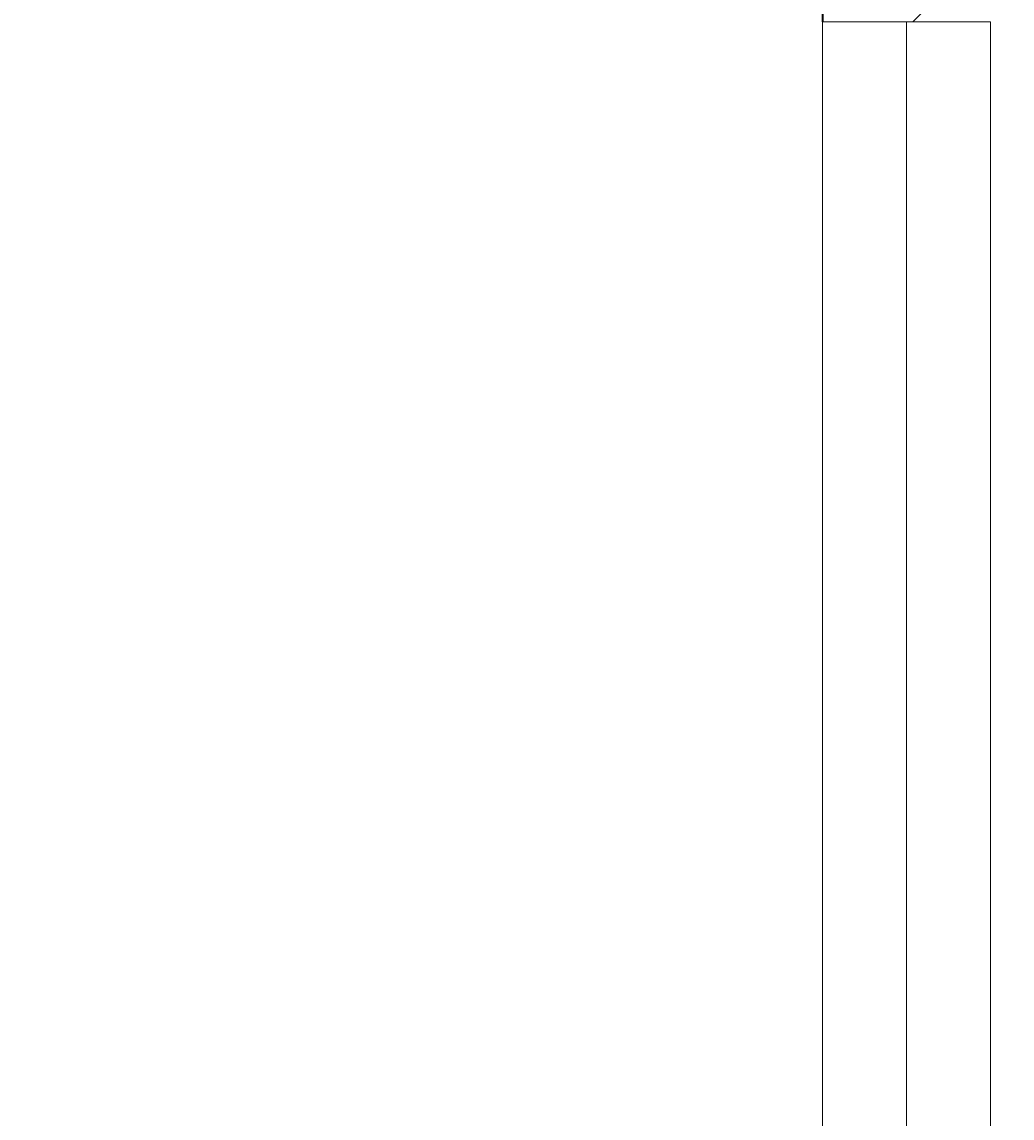
# Model space of a CAD drawing. Units: inches. Extents: x 1885 to 2748, y 783 to 2421.
# Tile 62 of 117: x 1995 to 2022, y 1949 to 1979. Entities that reach past the tile are written whole.
import ezdxf

# ---------------------------------------------------------------- set-up
doc = ezdxf.new("R2010")
doc.units = ezdxf.units.IN
for name, color, linetype, lineweight in [('A-ANNO-DIMS', 2, 'Continuous', 18), ('A-GLAZ', 181, 'Continuous', 18), ('A-WALL', 7, 'Continuous', 35)]:
    doc.layers.add(name, color=color, linetype=linetype, lineweight=lineweight)
doc.layers.add('A-WALL-PATT', color=85, linetype='Continuous', lineweight=13, true_color=0x58ba48)
doc.styles.get("Standard").update_dxf_attribs({"font": 'arial.ttf'})
doc.dimstyles.get("Standard").update_dxf_attribs({"dimtxt": 0.18, "dimasz": 0.18, "dimexe": 0.18, "dimexo": 0.0625, "dimgap": 0.09, "dimtad": 0, "dimtih": 1, "dimtoh": 1, "dimdec": 4, "dimzin": 0, "dimdsep": 46, "dimtxsty": 'Standard', "dimcen": 0.09, "dimadec": 0, "dimazin": 0, "dimtfac": 1, "dimtdec": 4, "dimtofl": 0, "dimtmove": 0, "dimatfit": 3, "dimfxl": 1, "dimtolj": 1, "dimtzin": 0, "dimarcsym": 0})

# ---------------------------------------------------------------- blocks, each defined once
blk = doc.blocks.new('WIN-60-ALT')
for p, q in [((0.004, 59.998), (4.504, 59.998)), ((0.004, 59.998), (0.004, -0.002)), ((4.504, 59.998), (2.254, 59.998)), ((2.254, 59.998), (2.254, -0.002)), ((4.504, -0.002), (4.504, 59.998))]:
    blk.add_line(p, q)
blk = doc.blocks.new('*D48')
at = {"layer": 'A-ANNO-DIMS', "color": 0, "lineweight": -2, "transparency": 16777216}
for p, q in [((1980.711, 2348.006), (1902.844, 2348.006)), ((1903.024, 2347.826), (1903.024, 2114.937)), ((1903.024, 1881.686), (1903.024, 2114.574)), ((2016.711, 1881.506), (1902.844, 1881.506))]:
    blk.add_line(p, q, dxfattribs=at)
at = {"layer": 'A-ANNO-DIMS', "color": 0, "transparency": 16777216}
for points in [[(1902.994, 2347.826), (1903.054, 2347.826), (1903.024, 2348.006)], [(1902.994, 1881.686), (1903.054, 1881.686), (1903.024, 1881.506)]]:
    blk.add_solid(points, dxfattribs=at)
at = {"layer": 'Defpoints', "color": 0, "transparency": 16777216}
for p in [(1903.024, 2348.006), (1980.774, 2348.006), (2016.774, 1881.506)]:
    blk.add_point(p, dxfattribs=at)
at = {"layer": 'A-ANNO-DIMS', "color": 0, "transparency": 16777216, "insert": (1903.024, 2114.756), "char_height": 0.18, "attachment_point": 5}
blk.add_mtext('\\A1;466.5', dxfattribs=at)

msp = doc.modelspace()

# ---------------------------------------------------------------- hatches: boundary and pattern name
at = {"layer": 'A-WALL-PATT'}
h = msp.add_hatch(dxfattribs=at)
h.set_pattern_fill('ANSI32', color=256)
h.paths.add_polyline_path([(2007.772, 2318.006), (1980.774, 2318.006), (1980.774, 2281.215), (1985.274, 2281.215), (1985.274, 2313.506), (2007.772, 2313.506), (2007.772, 2315.756)])
h.paths.add_polyline_path([(2094.324, 2318.006), (2067.772, 2318.006), (2067.772, 2313.506), (2094.324, 2313.506), (2094.324, 2315.756)])
h.paths.add_polyline_path([(2131.367, 2315.756), (2131.367, 2318.006), (2131.189, 2318.006), (2112.609, 2318.006), (2112.609, 2313.506), (2117.274, 2313.506), (2117.274, 2255.201), (2121.774, 2255.201), (2121.774, 2313.506), (2131.367, 2313.506)])
h.paths.add_polyline_path([(2190.512, 2318.006), (2155.367, 2318.006), (2155.367, 2313.506), (2169.774, 2313.506), (2169.774, 2229.506), (2121.774, 2229.506), (2121.774, 2233.451), (2119.524, 2233.451), (2117.274, 2233.451), (2117.274, 2201.101), (2121.774, 2201.101), (2121.774, 2225.006), (2169.774, 2225.006), (2169.774, 2165.006), (2306.274, 2165.006), (2306.274, 2066.006), (2310.774, 2066.006), (2344.274, 2066.006), (2486.274, 2066.006), (2486.274, 1886.006), (2483.02, 1886.006), (2483.02, 1881.506), (2486.274, 1881.506), (2486.274, 1880.678), (2490.774, 1880.678), (2490.774, 2070.506), (2344.274, 2070.506), (2310.774, 2070.506), (2310.774, 2165.006), (2310.774, 2173.636), (2308.524, 2173.636), (2306.274, 2173.636), (2306.274, 2169.506), (2174.274, 2169.506), (2174.274, 2313.506), (2190.512, 2313.506), (2190.512, 2315.756)])
h.paths.add_polyline_path([(1985.274, 2221.215), (1980.774, 2221.215), (1980.774, 2165.006), (1992.774, 2165.006), (1992.774, 2141.927), (1997.274, 2141.927), (1997.274, 2165.006), (2117.274, 2165.006), (2117.274, 2163.126), (2121.774, 2163.126), (2121.774, 2172.734), (2119.524, 2172.734), (2117.274, 2172.734), (2117.274, 2169.506), (1985.274, 2169.506)])
h.paths.add_polyline_path([(1997.274, 2105.927), (1992.774, 2105.927), (1992.774, 2070.506), (2016.774, 2070.506), (2016.774, 2059.123), (2019.024, 2059.123), (2021.274, 2059.123), (2021.274, 2070.506), (2117.274, 2070.506), (2117.274, 2022.506), (2114.423, 2022.506), (2114.423, 2018.006), (2123.627, 2018.006), (2123.627, 2020.256), (2123.627, 2022.506), (2121.774, 2022.506), (2121.774, 2142.587), (2119.524, 2142.587), (2117.274, 2142.587), (2117.274, 2075.006), (1997.274, 2075.006)])
h.paths.add_polyline_path([(2092.029, 2020.256), (2092.029, 2022.506), (2021.274, 2022.506), (2021.274, 2035.123), (2016.774, 2035.123), (2016.774, 2018.006), (2016.774, 1978.784), (2021.274, 1978.784), (2021.274, 2018.006), (2092.029, 2018.006)])
h.paths.add_polyline_path([(2260.938, 2022.506), (2153.105, 2022.506), (2153.105, 2020.256), (2153.105, 2018.006), (2155.274, 2018.006), (2155.274, 1886.006), (2107.629, 1886.006), (2107.629, 1881.506), (2182.911, 1881.506), (2182.911, 1883.756), (2182.911, 1886.006), (2159.774, 1886.006), (2159.774, 2018.006), (2260.938, 2018.006), (2260.938, 2020.256)])
h.paths.add_polyline_path([(2047.629, 1883.756), (2047.629, 1886.006), (2021.274, 1886.006), (2021.274, 1918.784), (2019.024, 1918.784), (2016.774, 1918.784), (2016.774, 1881.506), (2047.629, 1881.506)])
h.paths.add_polyline_path([(2306.361, 1883.756), (2306.361, 1886.006), (2296.274, 1886.006), (2296.274, 1982.006), (2316.535, 1982.006), (2316.535, 1984.256), (2316.535, 1986.506), (2296.274, 1986.506), (2296.274, 2022.506), (2289.276, 2022.506), (2289.276, 2018.006), (2291.774, 2018.006), (2291.774, 1886.006), (2242.911, 1886.006), (2242.911, 1881.506), (2306.361, 1881.506)], flags=17)
h.paths.add_polyline_path([(1985.274, 1843.006), (2021.6, 1843.006), (2021.534, 1845.441), (2021.477, 1847.506), (1980.774, 1847.506), (1980.774, 1809.446), (1985.274, 1809.446)])
h.paths.add_polyline_path([(2131.482, 1845.256), (2131.482, 1847.506), (2081.534, 1847.506), (2081.534, 1843.006), (2117.274, 1843.006), (2117.274, 1784.147), (2119.524, 1784.147), (2121.774, 1784.147), (2121.774, 1843.006), (2131.482, 1843.006)])
h.paths.add_polyline_path([(2203.886, 1847.506), (2155.482, 1847.506), (2155.482, 1843.006), (2169.774, 1843.006), (2169.774, 1759.006), (2121.774, 1759.006), (2121.774, 1761.457), (2117.274, 1761.457), (2117.274, 1730.429), (2121.774, 1730.429), (2121.774, 1754.506), (2177.421, 1754.506), (2177.421, 1756.756), (2177.421, 1759.006), (2174.274, 1759.006), (2174.274, 1843.006), (2203.886, 1843.006)])
h.paths.add_polyline_path([(2335.554, 1845.256), (2335.554, 1847.506), (2239.886, 1847.506), (2239.886, 1843.006), (2306.274, 1843.006), (2306.274, 1759.006), (2199.486, 1759.006), (2199.486, 1754.506), (2310.774, 1754.506), (2310.774, 1843.006), (2335.554, 1843.006)])
h.paths.add_polyline_path([(2348.774, 2022.506), (2344.274, 2022.506), (2344.274, 1986.506), (2341.681, 1986.506), (2341.681, 1982.006), (2344.274, 1982.006), (2344.274, 1886.006), (2330.361, 1886.006), (2330.361, 1881.506), (2361.627, 1881.506), (2361.627, 1883.756), (2361.627, 1886.006), (2348.774, 1886.006)], flags=17)
h.paths.add_polyline_path([(2283.251, 2315.756), (2283.251, 2318.006), (2238.512, 2318.006), (2238.512, 2313.506), (2283.251, 2313.506)], flags=17)
h.paths.add_polyline_path([(2363.274, 2348.006), (2388.677, 2348.006), (2388.677, 2350.256), (2388.677, 2352.506), (2358.774, 2352.506), (2358.774, 2348.006), (2358.774, 2318.006), (2344.481, 2318.006), (2344.481, 2313.506), (2358.774, 2313.506), (2358.774, 2229.506), (2310.774, 2229.506), (2310.774, 2231.952), (2306.274, 2231.952), (2306.274, 2205.611), (2310.774, 2205.611), (2310.774, 2225.006), (2358.774, 2225.006), (2358.774, 2211.506), (2452.329, 2211.506), (2452.329, 2213.756), (2452.329, 2216.006), (2363.274, 2216.006), (2363.274, 2318.006)])
h.paths.add_polyline_path([(2310.774, 2313.506), (2320.481, 2313.506), (2320.481, 2315.756), (2320.481, 2318.006), (2302.728, 2318.006), (2302.728, 2313.506), (2306.274, 2313.506), (2306.274, 2251.076), (2310.774, 2251.076)], flags=17)
h.paths.add_polyline_path([(2490.774, 2352.506), (2486.274, 2352.506), (2448.677, 2352.506), (2448.677, 2348.006), (2486.274, 2348.006), (2486.274, 2318.006), (2486.274, 2216.006), (2481.78, 2216.006), (2481.78, 2211.506), (2486.274, 2211.506), (2486.274, 2165.006), (2493.289, 2165.006), (2493.289, 2167.256), (2493.289, 2169.506), (2490.774, 2169.506), (2490.774, 2313.506), (2494.429, 2313.506), (2494.429, 2318.006), (2490.774, 2318.006)])
h.paths.add_polyline_path([(2534.653, 2318.006), (2515.691, 2318.006), (2515.691, 2313.506), (2534.653, 2313.506), (2534.653, 2315.756)])
h.paths.add_polyline_path([(2618.274, 2318.006), (2594.653, 2318.006), (2594.653, 2313.506), (2613.774, 2313.506), (2613.774, 2281.706), (2618.274, 2281.706)])
h.paths.add_polyline_path([(2618.274, 2221.706), (2613.774, 2221.706), (2613.774, 2169.506), (2554.019, 2169.506), (2554.019, 2165.006), (2613.774, 2165.006), (2613.774, 2152.878), (2618.274, 2152.878)])
h.paths.add_polyline_path([(2618.274, 2128.878), (2616.024, 2128.878), (2613.774, 2128.878), (2613.774, 2117.006), (2529.774, 2117.006), (2529.774, 2165.006), (2532.848, 2165.006), (2532.848, 2169.506), (2522.867, 2169.506), (2522.867, 2165.006), (2525.274, 2165.006), (2525.274, 2117.006), (2525.274, 2112.506), (2525.274, 2108.576), (2529.774, 2108.576), (2529.774, 2112.506), (2613.774, 2112.506), (2613.774, 2080.19), (2618.274, 2080.19)])
h.paths.add_polyline_path([(2618.274, 2044.19), (2616.024, 2044.19), (2613.774, 2044.19), (2613.774, 2015.506), (2529.774, 2015.506), (2529.774, 2088.582), (2527.524, 2088.582), (2525.274, 2088.582), (2525.274, 2011.006), (2613.774, 2011.006), (2613.774, 1956.755), (2618.274, 1956.755)])
h.paths.add_polyline_path([(2618.274, 1881.506), (2618.274, 1896.755), (2613.774, 1896.755), (2613.774, 1881.506), (2613.774, 1847.506), (2592.715, 1847.506), (2592.715, 1843.006), (2613.774, 1843.006), (2613.774, 1765.006), (2613.774, 1760.506), (2609.621, 1760.506), (2609.621, 1756.006), (2613.774, 1756.006), (2613.774, 1660.006), (2608.544, 1660.006), (2608.544, 1655.506), (2613.774, 1655.506), (2613.774, 1508.158), (2618.274, 1508.158)])
h.paths.add_polyline_path([(2565.774, 1843.006), (2568.997, 1843.006), (2568.997, 1847.506), (2490.774, 1847.506), (2490.774, 1849.7), (2488.524, 1849.7), (2486.274, 1849.7), (2486.274, 1847.506), (2477.274, 1847.506), (2477.274, 1838.506), (2477.274, 1821.493), (2486.274, 1821.493), (2486.274, 1838.506), (2561.274, 1838.506), (2561.274, 1765.006), (2486.274, 1765.006), (2486.274, 1786.157), (2477.274, 1786.157), (2477.274, 1765.006), (2477.274, 1756.006), (2486.274, 1756.006), (2565.774, 1756.006), (2585.621, 1756.006), (2585.621, 1758.256), (2585.621, 1760.506), (2565.774, 1760.506), (2565.774, 1765.006)])
h.paths.add_polyline_path([(2486.274, 1651.006), (2561.274, 1651.006), (2561.274, 1567.006), (2486.274, 1567.006), (2486.274, 1591.321), (2477.274, 1591.321), (2477.274, 1567.006), (2477.274, 1558.006), (2477.274, 1555.439), (2481.774, 1555.439), (2481.774, 1558.006), (2568.653, 1558.006), (2568.653, 1560.256), (2568.653, 1562.506), (2565.774, 1562.506), (2565.774, 1655.506), (2584.544, 1655.506), (2584.544, 1657.756), (2584.544, 1660.006), (2565.774, 1660.006), (2486.274, 1660.006), (2477.274, 1660.006), (2477.274, 1651.006), (2477.274, 1632.989), (2486.274, 1632.989)])
h.paths.add_polyline_path([(2449.967, 1883.756), (2449.967, 1886.006), (2421.627, 1886.006), (2421.627, 1881.506), (2449.967, 1881.506)], flags=17)
h.paths.add_polyline_path([(2447.274, 1847.506), (2395.554, 1847.506), (2395.554, 1843.006), (2442.774, 1843.006), (2442.774, 1809.27), (2447.274, 1809.27)])
h.paths.add_polyline_path([(1985.274, 1749.446), (1980.774, 1749.446), (1980.774, 1694.504), (1985.274, 1694.504), (1985.274, 1694.506), (1986.897, 1694.506), (1986.897, 1697.78), (1986.897, 1699.006), (1985.274, 1699.006)])
h.paths.add_polyline_path([(2152.774, 1699.006), (2121.774, 1699.006), (2121.774, 1703.668), (2119.524, 1703.668), (2117.274, 1703.668), (2117.274, 1699.006), (2009.219, 1699.006), (2009.219, 1694.506), (2148.274, 1694.506), (2148.274, 1692.631), (2152.774, 1692.631)])
h.paths.add_polyline_path([(2016.274, 1694.506), (2011.774, 1694.506), (2011.774, 1558.006), (2040.806, 1558.006), (2040.806, 1560.256), (2040.806, 1562.506), (2016.274, 1562.506)])
h.paths.add_polyline_path([(2152.774, 1663.017), (2150.524, 1663.017), (2148.274, 1663.017), (2148.274, 1562.506), (2100.806, 1562.506), (2100.806, 1558.006), (2165.119, 1558.006), (2165.119, 1560.256), (2165.119, 1562.506), (2152.774, 1562.506), (2152.774, 1610.506), (2224.774, 1610.506), (2224.774, 1607.99), (2229.274, 1607.99), (2229.274, 1615.006), (2152.774, 1615.006)])
h.paths.add_polyline_path([(2238.613, 1560.256), (2238.613, 1562.506), (2229.274, 1562.506), (2229.274, 1588.756), (2227.024, 1588.763), (2224.774, 1588.771), (2224.774, 1562.506), (2189.119, 1562.506), (2189.119, 1558.006), (2238.613, 1558.006)])
h.paths.add_polyline_path([(2336.024, 1560.256), (2336.024, 1562.506), (2310.774, 1562.506), (2310.774, 1656.347), (2308.524, 1656.347), (2306.274, 1656.347), (2306.274, 1562.506), (2286.613, 1562.506), (2286.613, 1558.006), (2336.024, 1558.006)])
h.paths.add_polyline_path([(2447.274, 1690.968), (2445.024, 1690.968), (2442.774, 1690.968), (2442.774, 1687.006), (2306.274, 1687.006), (2306.274, 1680.75), (2310.774, 1680.75), (2310.774, 1682.506), (2442.774, 1682.506), (2442.774, 1562.506), (2396.024, 1562.506), (2396.024, 1558.006), (2447.274, 1558.006)])
h.paths.add_polyline_path([(2447.274, 1749.27), (2445.024, 1749.27), (2442.774, 1749.27), (2442.774, 1717.232), (2447.274, 1717.232)])
h.paths.add_polyline_path([(2044.674, 1521.756), (2044.674, 1524.006), (2007.274, 1524.006), (2007.274, 1503.49), (2009.524, 1503.49), (2011.774, 1503.49), (2011.774, 1519.506), (2044.674, 1519.506)])
h.paths.add_polyline_path([(2177.969, 1521.756), (2177.969, 1524.006), (2104.674, 1524.006), (2104.674, 1519.506), (2145.774, 1519.506), (2145.774, 1387.506), (2143.37, 1387.506), (2143.37, 1383.006), (2251.585, 1383.006), (2251.585, 1385.256), (2251.585, 1387.506), (2150.274, 1387.506), (2150.274, 1519.506), (2177.969, 1519.506)])
h.paths.add_polyline_path([(2298.704, 1524.006), (2237.969, 1524.006), (2237.969, 1519.506), (2282.274, 1519.506), (2282.274, 1387.506), (2279.683, 1387.506), (2279.683, 1383.006), (2286.774, 1383.006), (2286.774, 1419.006), (2312.451, 1419.006), (2312.451, 1421.256), (2312.451, 1423.506), (2286.774, 1423.506), (2286.774, 1519.506), (2298.704, 1519.506), (2298.704, 1521.722)], flags=17)
h.paths.add_polyline_path([(2361.897, 1521.756), (2361.897, 1524.006), (2322.704, 1524.006), (2322.704, 1519.506), (2334.774, 1519.506), (2334.774, 1423.506), (2331.93, 1423.506), (2331.93, 1419.006), (2334.774, 1419.006), (2334.774, 1387.506), (2334.774, 1383.228), (2339.274, 1383.228), (2339.274, 1387.506), (2339.274, 1519.506), (2361.897, 1519.506)], flags=17)
h.paths.add_polyline_path([(2447.274, 1521.756), (2447.274, 1524.006), (2421.897, 1524.006), (2421.897, 1519.506), (2447.274, 1519.506)], flags=17)
h.paths.add_polyline_path([(2481.774, 1529.6), (2479.524, 1529.6), (2477.274, 1529.6), (2477.274, 1524.006), (2474.489, 1524.006), (2474.489, 1519.506), (2477.274, 1519.506), (2477.274, 1334.506), (2296.774, 1334.506), (2296.774, 1240.506), (2160.274, 1240.506), (2160.274, 1180.506), (2112.274, 1180.506), (2112.274, 1207.692), (2110.024, 1207.692), (2107.774, 1207.692), (2107.774, 1171.609), (2112.274, 1171.609), (2112.274, 1176.006), (2160.274, 1176.006), (2160.274, 1092.006), (2144.221, 1092.006), (2144.221, 1087.506), (2189.497, 1087.506), (2189.497, 1089.756), (2189.497, 1092.006), (2164.774, 1092.006), (2164.774, 1236.006), (2296.774, 1236.006), (2296.774, 1231.912), (2301.274, 1231.912), (2301.274, 1330.006), (2481.774, 1330.006), (2481.774, 1387.506)])
h.paths.add_polyline_path([(2618.274, 1448.158), (2613.774, 1448.158), (2613.774, 1382.506), (2529.774, 1382.506), (2525.274, 1382.506), (2525.274, 1307.062), (2529.774, 1307.062), (2529.774, 1378.006), (2613.774, 1378.006), (2613.774, 1354.988), (2618.274, 1354.988)])
h.paths.add_polyline_path([(2618.274, 1318.988), (2613.774, 1318.988), (2613.774, 1281.006), (2529.774, 1281.006), (2529.774, 1283.786), (2527.524, 1283.786), (2525.274, 1283.786), (2525.274, 1228.506), (2516.794, 1228.506), (2516.794, 1224.006), (2533.484, 1224.006), (2533.484, 1226.256), (2533.484, 1228.506), (2529.774, 1228.506), (2529.774, 1276.506), (2613.774, 1276.506), (2613.774, 1266.02), (2618.274, 1266.02)])
h.paths.add_polyline_path([(2618.274, 1134.964), (2613.774, 1134.964), (2613.774, 1092.006), (2594.545, 1092.006), (2594.545, 1087.506), (2618.274, 1087.506)])
h.paths.add_polyline_path([(2534.545, 1092.006), (2509.765, 1092.006), (2509.765, 1087.506), (2534.545, 1087.506), (2534.545, 1089.756)])
h.paths.add_polyline_path([(2481.274, 1224.006), (2484.117, 1224.006), (2484.117, 1226.256), (2484.117, 1228.506), (2476.774, 1228.506), (2476.774, 1198.506), (2471.61, 1198.506), (2471.61, 1194.006), (2476.774, 1194.006), (2476.774, 1062.006), (2436.894, 1062.006), (2436.894, 1057.506), (2476.774, 1057.506), (2481.274, 1057.506), (2481.274, 1062.006), (2481.274, 1087.506), (2485.354, 1087.506), (2485.354, 1089.756), (2485.354, 1092.006), (2481.274, 1092.006), (2481.274, 1117.506)])
h.paths.add_polyline_path([(2439.898, 1198.506), (2349.274, 1198.506), (2349.274, 1194.006), (2349.274, 1180.506), (2301.274, 1180.506), (2301.274, 1201.896), (2299.024, 1201.896), (2296.774, 1201.896), (2296.774, 1172.335), (2299.024, 1172.335), (2301.274, 1172.335), (2301.274, 1176.006), (2349.274, 1176.006), (2349.274, 1092.006), (2334.452, 1092.006), (2334.452, 1087.506), (2349.274, 1087.506), (2349.274, 1057.506), (2353.774, 1057.506), (2376.894, 1057.506), (2376.894, 1059.756), (2376.894, 1062.006), (2353.774, 1062.006), (2353.774, 1087.506), (2353.774, 1180.506), (2353.774, 1194.006), (2439.898, 1194.006), (2439.898, 1196.256)])
h.paths.add_polyline_path([(2270.596, 1089.756), (2270.596, 1092.006), (2249.497, 1092.006), (2249.497, 1087.506), (2270.596, 1087.506)], flags=17)
h.paths.add_polyline_path([(2310.452, 1092.006), (2301.274, 1092.006), (2301.274, 1153.292), (2296.774, 1153.292), (2296.774, 1092.006), (2293.786, 1092.006), (2293.786, 1087.506), (2310.452, 1087.506), (2310.452, 1089.756)], flags=17)
h.paths.add_polyline_path([(2112.274, 1150.328), (2110.024, 1150.328), (2107.774, 1150.328), (2107.774, 1092.006), (2104.465, 1092.006), (2104.465, 1087.506), (2120.221, 1087.506), (2120.221, 1089.756), (2120.221, 1092.006), (2112.274, 1092.006)])
h.paths.add_polyline_path([(2082.172, 1092.006), (2058.144, 1092.006), (2058.144, 1087.506), (2082.172, 1087.506), (2082.172, 1089.756)])
h.paths.add_polyline_path([(1975.774, 1145.638), (1971.274, 1145.638), (1971.274, 1087.506), (1980.774, 1087.506), (1998.144, 1087.506), (1998.144, 1089.756), (1998.144, 1092.006), (1985.274, 1092.006), (1975.774, 1092.006)])
h.paths.add_polyline_path([(2112.274, 1244.385), (2110.024, 1244.385), (2107.774, 1244.385), (2107.774, 1240.506), (1992.274, 1240.506), (1992.274, 1271.008), (1987.774, 1271.008), (1987.774, 1240.506), (1980.774, 1240.506), (1975.774, 1240.506), (1971.274, 1240.506), (1971.274, 1205.638), (1975.774, 1205.638), (1975.774, 1236.006), (2107.774, 1236.006), (2107.774, 1233.444), (2112.274, 1233.444), (2112.274, 1236.006)])
h.paths.add_polyline_path([(2112.274, 1383.006), (2114.783, 1383.006), (2114.783, 1385.256), (2114.783, 1387.506), (2102.476, 1387.506), (2102.476, 1383.006), (2107.774, 1383.006), (2107.774, 1335.006), (2011.774, 1335.006), (2011.774, 1349.939), (2007.274, 1349.939), (2007.274, 1335.006), (1987.774, 1335.006), (1987.774, 1330.506), (1987.774, 1307.008), (1992.274, 1307.008), (1992.274, 1330.506), (2007.274, 1330.506), (2107.774, 1330.506), (2107.774, 1264.711), (2112.274, 1264.711)])
h.paths.add_polyline_path([(2077.857, 1387.506), (2011.774, 1387.506), (2011.774, 1390.036), (2009.524, 1390.036), (2007.274, 1390.036), (2007.274, 1373.939), (2011.774, 1373.939), (2011.774, 1383.006), (2077.857, 1383.006)])
h.paths.add_polyline_path([(2011.774, 1443.49), (2007.274, 1443.49), (2007.274, 1410.248), (2011.774, 1410.248)])

# ---------------------------------------------------------------- linework, layer by layer
at = {"layer": 'A-WALL'}
msp.add_line((2016.774, 2018.006), (2016.774, 1978.784), dxfattribs=at)

# ---------------------------------------------------------------- block references
at = {"layer": 'A-GLAZ'}
msp.add_blockref('WIN-60-ALT', (2016.77, 1918.787), dxfattribs=at)

# ---------------------------------------------------------------- dimensions: what is measured, and where the dimension line sits
at = {"layer": 'A-ANNO-DIMS'}
dim = msp.add_linear_dim(base=(1903.024, 2348.006), p1=(2016.774, 1881.506), p2=(1980.774, 2348.006), angle=90, dimstyle='Standard', override={"dimdec": 1, "dimlfac": 1, "dimrnd": 0, "dimzin": 0, "dimdsep": 46, "dimlunit": 2}, dxfattribs=at)
dim.commit()
dim.dimension.update_dxf_attribs({"geometry": '*D48', "text_midpoint": (1903.024, 2114.756)})

doc.saveas('drawing.dxf')
